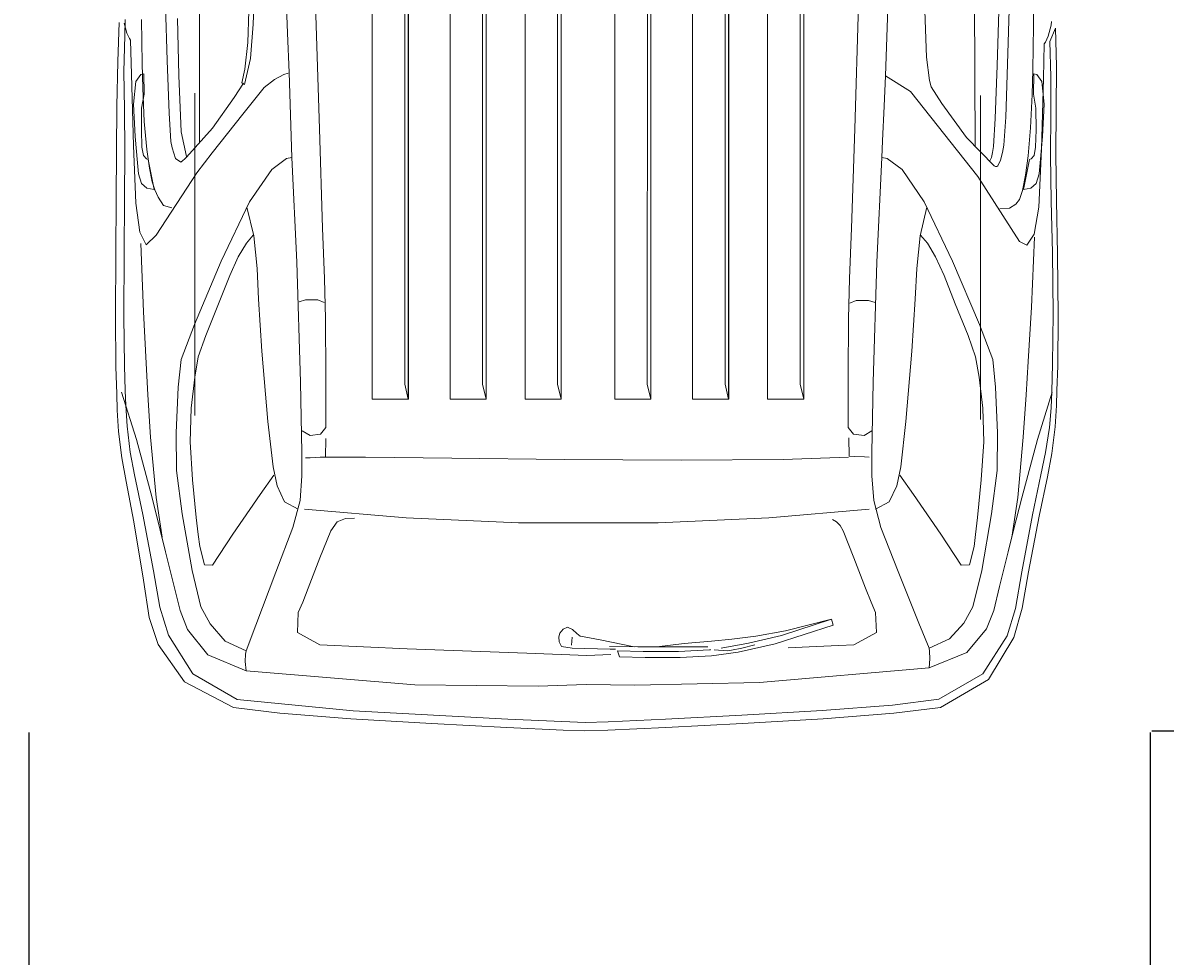
# Model space of a CAD drawing. Units: inches. Extents: x 37 to 706, y -568 to 110.
# Tile 3 of 24: x 126 to 171, y -450 to -413. Entities that reach past the tile are written whole.
import ezdxf

# ---------------------------------------------------------------- set-up
doc = ezdxf.new("R2010")
doc.units = ezdxf.units.IN
doc.header["$MEASUREMENT"] = 0
for name, color, linetype, lineweight in [('A-ANNO-DIMS', 2, 'Continuous', 18), ('A-SITE-VEHI', 8, 'Continuous', 13), ('A-WALL-PATT', 252, 'Continuous', 13)]:
    doc.layers.add(name, color=color, linetype=linetype, lineweight=lineweight)
doc.styles.get("Standard").update_dxf_attribs({"font": 'arial.ttf'})
doc.dimstyles.get("Standard").update_dxf_attribs({"dimtxt": 0.18, "dimasz": 0.18, "dimexe": 0.18, "dimexo": 0.0625, "dimgap": 0.09, "dimtad": 0, "dimtih": 1, "dimtoh": 1, "dimdec": 0, "dimzin": 0, "dimdsep": 46, "dimlunit": 3, "dimtxsty": 'Standard', "dimcen": 0.09, "dimadec": 0, "dimazin": 0, "dimtfac": 1, "dimtdec": 0, "dimtofl": 0, "dimtmove": 0, "dimatfit": 3, "dimfxl": 1, "dimtolj": 1, "dimtzin": 0, "dimarcsym": 0})

# ---------------------------------------------------------------- blocks, each defined once
blk = doc.blocks.new('CAR-SEDAN-PLAN')
for p, q in [((13.604, 13.133), (13.604, 50.661)), ((14.891, 13.73), (14.905, 50.543)), ((15.034, 50.661), (15.034, 13.133)), ((15.035, 50.661), (15.035, 13.133)), ((16.686, 13.133), (16.686, 50.661)), ((17.973, 13.73), (17.987, 50.543)), ((18.115, 50.661), (18.115, 13.133)), ((18.117, 50.661), (18.117, 13.133)), ((19.657, 13.133), (19.657, 50.661)), ((20.944, 13.73), (20.958, 50.543)), ((21.087, 50.661), (21.087, 13.133)), ((21.088, 50.661), (21.088, 13.133)), ((23.212, 13.133), (23.212, 50.661)), ((24.499, 13.73), (24.513, 50.543)), ((24.642, 50.661), (24.642, 13.133)), ((24.643, 50.661), (24.643, 13.133)), ((26.294, 13.133), (26.294, 50.661)), ((27.581, 13.73), (27.595, 50.543)), ((27.723, 50.661), (27.723, 13.133)), ((27.725, 50.661), (27.725, 13.133)), ((29.265, 13.133), (29.265, 50.661)), ((30.553, 13.73), (30.567, 50.543)), ((30.696, 50.661), (30.696, 13.133)), ((34.17, 32.694), (34.002, 27.855)), ((10.065, 32.102), (10.25, 27.635)), ((6.755, 31.469), (6.762, 26.153)), ((39.857, 31.627), (39.796, 27.924)), ((37.457, 31.221), (37.48, 25.971)), ((5.415, 28.71), (5.486, 26.554)), ((8.919, 28.667), (8.894, 27.992)), ((11.511, 23.847), (11.355, 28.753)), ((32.718, 23.847), (32.874, 28.753)), ((35.501, 28.522), (35.566, 26.682)), ((38.84, 28.558), (38.769, 26.402)), ((3.52, 26.505), (3.579, 28.059)), ((3.815, 28.178), (3.801, 27.531)), ((4.464, 28.172), (4.492, 26.437)), ((5.892, 28.219), (5.946, 25.954)), ((8.671, 27.267), (8.713, 28.508)), ((38.427, 28.503), (38.356, 26.347)), ((40.498, 27.951), (40.519, 28.091)), ((3.88, 27.64), (3.771, 28.026)), ((3.984, 27.426), (3.88, 27.64)), ((8.894, 27.992), (8.788, 26.636)), ((10.25, 27.635), (10.317, 26.081)), ((34.002, 27.855), (33.939, 25.939)), ((39.796, 27.924), (39.768, 26.188)), ((40.387, 27.519), (40.498, 27.951)), ((40.449, 27.298), (40.675, 27.828)), ((40.675, 27.828), (40.709, 26.308)), ((3.801, 27.531), (3.77, 26.116)), ((4.03, 27.36), (3.984, 27.426)), ((4.062, 25.992), (4.03, 27.36)), ((8.558, 26.208), (8.671, 27.267)), ((40.194, 25.84), (40.225, 27.208)), ((40.225, 27.208), (40.276, 27.281)), ((40.276, 27.281), (40.387, 27.519)), ((40.488, 25.901), (40.449, 27.298)), ((3.484, 24.748), (3.52, 26.505)), ((4.492, 26.437), (4.514, 25.45)), ((5.486, 26.554), (5.557, 24.461)), ((8.788, 26.636), (8.548, 25.606)), ((35.566, 26.682), (35.686, 25.757)), ((38.356, 26.347), (38.285, 24.254)), ((38.769, 26.402), (38.698, 24.309)), ((40.709, 26.308), (40.697, 24.613)), ((3.77, 26.116), (3.787, 24.613)), ((4.141, 23.187), (4.062, 25.992)), ((4.44, 26.001), (4.24, 25.718)), ((4.551, 26.018), (4.44, 26.001)), ((4.571, 25.221), (4.551, 26.018)), ((5.946, 25.954), (6.033, 23.727)), ((6.762, 26.153), (6.765, 23.311)), ((8.437, 25.661), (8.558, 26.208)), ((9.729, 25.804), (9.322, 25.478)), ((10.107, 25.994), (9.729, 25.804)), ((10.273, 26.055), (10.107, 25.994)), ((10.317, 26.081), (10.426, 22.71)), ((33.939, 25.939), (33.885, 24.736)), ((33.939, 25.939), (34.933, 25.326)), ((37.48, 25.971), (37.49, 23.159)), ((39.768, 26.188), (39.746, 25.202)), ((39.796, 25.221), (39.816, 26.018)), ((39.816, 26.018), (39.928, 26.001)), ((39.928, 26.001), (40.128, 25.718)), ((40.115, 23.036), (40.194, 25.84)), ((40.485, 24.433), (40.488, 25.901)), ((4.24, 25.718), (4.151, 24.827)), ((4.514, 25.45), (4.576, 24.132)), ((8.505, 25.655), (8.139, 25.088)), ((8.548, 25.606), (8.437, 25.661)), ((9.322, 25.478), (8.474, 24.429)), ((35.686, 25.757), (35.75, 25.503)), ((35.75, 25.503), (36.174, 24.851)), ((40.128, 25.718), (40.217, 24.827)), ((4.47, 24.664), (4.571, 25.221)), ((6.579, 25.262), (6.579, 12.495)), ((8.139, 25.088), (7.271, 23.868)), ((34.933, 25.326), (37.597, 21.952)), ((37.699, 25.17), (37.699, 12.334)), ((39.746, 25.202), (39.684, 23.884)), ((39.897, 24.664), (39.796, 25.221)), ((3.472, 22.96), (3.484, 24.748)), ((3.787, 24.613), (3.803, 22.96)), ((4.151, 24.827), (4.216, 23.545)), ((4.466, 23.8), (4.47, 24.664)), ((5.557, 24.461), (5.628, 23.347)), ((33.885, 24.736), (33.823, 23.365)), ((36.174, 24.851), (37.15, 23.504)), ((39.901, 23.8), (39.897, 24.664)), ((40.217, 24.827), (40.151, 23.545)), ((40.697, 24.613), (40.683, 22.854)), ((4.576, 24.132), (4.669, 23.027)), ((8.474, 24.429), (7.27, 22.892)), ((38.285, 24.254), (38.214, 23.14)), ((38.698, 24.309), (38.627, 23.195)), ((40.477, 22.799), (40.485, 24.433)), ((4.216, 23.545), (4.303, 22.495)), ((4.482, 23.116), (4.466, 23.8)), ((6.033, 23.727), (6.25, 22.744)), ((7.271, 23.868), (6.252, 22.718)), ((11.64, 19.914), (11.511, 23.847)), ((32.59, 19.914), (32.718, 23.847)), ((39.684, 23.884), (39.591, 22.779)), ((39.885, 23.116), (39.901, 23.8)), ((40.151, 23.545), (40.064, 22.495)), ((4.243, 20.896), (4.141, 23.187)), ((4.546, 22.789), (4.482, 23.116)), ((5.628, 23.347), (5.675, 23.096)), ((5.675, 23.096), (5.809, 22.664)), ((33.823, 23.365), (33.793, 22.71)), ((37.15, 23.504), (38.236, 22.378)), ((38.214, 23.14), (38.178, 22.908)), ((38.627, 23.195), (38.57, 22.906)), ((39.821, 22.789), (39.885, 23.116)), ((3.463, 21.075), (3.472, 22.96)), ((3.803, 22.96), (3.793, 21.075)), ((4.666, 22.658), (4.546, 22.789)), ((4.73, 22.634), (4.666, 22.658)), ((4.669, 23.027), (4.776, 22.289)), ((4.964, 21.437), (4.73, 22.634)), ((5.809, 22.664), (6.019, 22.53)), ((6.095, 22.587), (6.173, 22.65)), ((6.173, 22.65), (6.252, 22.718)), ((7.27, 22.892), (6.658, 22.104)), ((10.213, 22.669), (9.627, 22.239)), ((10.426, 22.71), (10.213, 22.669)), ((10.426, 22.71), (10.623, 18.569)), ((33.793, 22.71), (33.596, 18.569)), ((33.793, 22.71), (34.007, 22.669)), ((34.007, 22.669), (34.593, 22.239)), ((38.142, 22.707), (38.056, 22.552)), ((38.178, 22.908), (38.142, 22.707)), ((38.57, 22.906), (38.496, 22.598)), ((39.404, 21.437), (39.637, 22.634)), ((39.591, 22.779), (39.479, 22.007)), ((39.637, 22.634), (39.702, 22.658)), ((39.702, 22.658), (39.821, 22.789)), ((40.012, 20.744), (40.115, 23.036)), ((40.502, 20.982), (40.477, 22.799)), ((40.683, 22.854), (40.709, 20.996)), ((4.303, 22.495), (4.347, 22.059)), ((4.776, 22.289), (4.883, 21.74)), ((6.019, 22.53), (6.095, 22.587)), ((9.627, 22.239), (8.747, 20.959)), ((34.593, 22.239), (35.473, 20.959)), ((38.236, 22.378), (38.293, 22.351)), ((38.293, 22.351), (38.344, 22.355)), ((38.344, 22.355), (38.389, 22.385)), ((38.496, 22.598), (38.389, 22.385)), ((40.064, 22.495), (40.02, 22.059)), ((4.347, 22.059), (4.458, 21.676)), ((4.883, 21.74), (4.989, 21.429)), ((6.658, 22.104), (5.04, 19.635)), ((37.597, 21.952), (39.239, 19.387)), ((39.479, 22.007), (39.364, 21.397)), ((40.02, 22.059), (39.909, 21.676)), ((4.458, 21.676), (4.673, 21.491)), ((4.673, 21.491), (4.964, 21.437)), ((4.989, 21.429), (5.122, 21.136)), ((39.364, 21.397), (39.252, 21.052)), ((39.695, 21.491), (39.404, 21.437)), ((39.909, 21.676), (39.695, 21.491)), ((3.446, 18.903), (3.463, 21.075)), ((3.793, 21.075), (3.776, 18.903)), ((4.396, 19.749), (4.243, 20.896)), ((5.122, 21.136), (5.335, 20.805)), ((8.747, 20.959), (7.622, 18.6)), ((35.473, 20.959), (36.598, 18.6)), ((39.099, 20.862), (38.843, 20.707)), ((39.252, 21.052), (39.099, 20.862)), ((40.548, 18.939), (40.502, 20.982)), ((40.709, 20.996), (40.757, 18.876)), ((5.335, 20.805), (5.672, 20.722)), ((8.64, 20.745), (8.911, 19.602)), ((35.58, 20.745), (35.309, 19.602)), ((38.843, 20.707), (38.468, 20.681)), ((39.822, 19.677), (40.012, 20.744)), ((11.712, 17.922), (11.64, 19.914)), ((32.517, 17.922), (32.59, 19.914)), ((4.655, 19.245), (4.396, 19.749)), ((5.04, 19.635), (4.655, 19.245)), ((8.89, 19.637), (8.625, 19.316)), ((8.911, 19.602), (9.047, 18.315)), ((35.309, 19.602), (35.172, 18.315)), ((35.33, 19.637), (35.595, 19.316)), ((39.532, 19.233), (39.822, 19.677)), ((39.844, 19.553), (39.718, 16.784)), ((4.434, 19.305), (4.545, 16.6)), ((8.625, 19.316), (8.297, 18.78)), ((35.595, 19.316), (35.923, 18.78)), ((39.239, 19.387), (39.532, 19.233)), ((3.437, 16.422), (3.446, 18.903)), ((3.776, 18.903), (3.767, 16.422)), ((7.622, 18.6), (6.561, 16.09)), ((8.297, 18.78), (7.961, 18.03)), ((10.623, 18.569), (10.765, 13.809)), ((33.596, 18.569), (33.455, 13.809)), ((35.923, 18.78), (36.259, 18.03)), ((36.598, 18.6), (37.659, 16.09)), ((40.573, 16.526), (40.548, 18.939)), ((40.757, 18.876), (40.783, 16.422)), ((9.047, 18.315), (9.104, 17.101)), ((35.172, 18.315), (35.115, 17.101)), ((7.961, 18.03), (7.517, 16.918)), ((11.752, 16.319), (11.712, 17.922)), ((32.477, 16.319), (32.517, 17.922)), ((36.259, 18.03), (36.702, 16.918)), ((7.517, 16.918), (7.011, 15.663)), ((9.104, 17.101), (9.236, 15.044)), ((10.707, 16.994), (10.967, 17.077)), ((10.967, 17.077), (11.449, 17.073)), ((11.449, 17.073), (11.705, 16.973)), ((32.78, 17.046), (32.525, 16.946)), ((33.262, 17.05), (32.78, 17.046)), ((33.522, 16.966), (33.262, 17.05)), ((35.115, 17.101), (34.983, 15.044)), ((36.702, 16.918), (37.209, 15.663)), ((39.718, 16.784), (39.589, 14.629)), ((3.453, 14.417), (3.437, 16.422)), ((3.767, 16.422), (3.785, 14.465)), ((4.545, 16.6), (4.646, 14.565)), ((11.771, 14.081), (11.752, 16.319)), ((32.458, 14.081), (32.477, 16.319)), ((40.555, 14.519), (40.573, 16.526)), ((40.783, 16.422), (40.764, 14.465)), ((6.561, 16.09), (6.031, 14.707)), ((37.659, 16.09), (38.188, 14.707)), ((7.011, 15.663), (6.71, 14.814)), ((37.209, 15.663), (37.509, 14.814)), ((9.236, 15.044), (9.472, 12.249)), ((34.983, 15.044), (34.748, 12.249)), ((4.646, 14.565), (4.709, 13.313)), ((6.031, 14.707), (5.922, 13.615)), ((6.71, 14.814), (6.571, 14.015)), ((37.509, 14.814), (37.648, 14.015)), ((38.188, 14.707), (38.298, 13.615)), ((39.589, 14.629), (39.51, 13.313)), ((40.522, 13.447), (40.555, 14.519)), ((3.483, 13.349), (3.453, 14.417)), ((3.785, 14.465), (3.82, 13.484)), ((11.772, 12.018), (11.771, 14.081)), ((32.458, 12.018), (32.458, 14.081)), ((40.764, 14.465), (40.73, 13.484)), ((5.922, 13.615), (5.844, 11.809)), ((6.571, 14.015), (6.432, 12.779)), ((10.765, 13.809), (10.819, 11.026)), ((15.034, 13.133), (14.891, 13.73)), ((18.115, 13.133), (17.973, 13.73)), ((21.087, 13.133), (20.944, 13.73)), ((24.642, 13.133), (24.499, 13.73)), ((27.723, 13.133), (27.581, 13.73)), ((30.696, 13.133), (30.553, 13.73)), ((33.455, 13.809), (33.4, 11.026)), ((37.648, 14.015), (37.787, 12.779)), ((38.298, 13.615), (38.376, 11.809)), ((3.499, 12.702), (3.483, 13.349)), ((3.673, 13.421), (4.262, 11.543)), ((3.82, 13.484), (3.838, 12.885)), ((4.709, 13.313), (4.826, 11.635)), ((15.035, 13.133), (13.604, 13.133)), ((18.117, 13.133), (16.686, 13.133)), ((21.088, 13.133), (19.657, 13.133)), ((24.643, 13.133), (23.212, 13.133)), ((27.725, 13.133), (26.294, 13.133)), ((30.696, 13.133), (29.265, 13.133)), ((39.51, 13.313), (39.394, 11.635)), ((40.546, 13.421), (39.958, 11.543)), ((40.504, 12.798), (40.522, 13.447)), ((40.73, 13.484), (40.711, 12.885)), ((3.552, 11.862), (3.499, 12.702)), ((3.838, 12.885), (3.891, 12.073)), ((6.432, 12.779), (6.389, 11.455)), ((37.787, 12.779), (37.831, 11.455)), ((40.436, 12.011), (40.504, 12.798)), ((40.711, 12.885), (40.658, 12.044)), ((9.472, 12.249), (9.676, 10.455)), ((34.748, 12.249), (34.544, 10.455)), ((3.686, 10.809), (3.552, 11.862)), ((3.891, 12.073), (4.021, 11.046)), ((5.844, 11.809), (5.853, 10.312)), ((10.833, 11.88), (11.14, 11.695)), ((11.56, 11.754), (11.772, 12.018)), ((32.669, 11.754), (32.458, 12.018)), ((33.396, 11.88), (33.089, 11.695)), ((38.376, 11.809), (38.367, 10.312)), ((40.277, 11.029), (40.436, 12.011)), ((40.658, 12.044), (40.524, 10.992)), ((4.262, 11.543), (4.883, 9.236)), ((4.826, 11.635), (5.045, 9.251)), ((6.389, 11.455), (6.488, 9.945)), ((11.14, 11.695), (11.56, 11.754)), ((11.772, 11.581), (11.748, 10.848)), ((32.479, 11.611), (32.503, 10.878)), ((33.089, 11.695), (32.669, 11.754)), ((37.831, 11.455), (37.732, 9.945)), ((39.394, 11.635), (39.174, 9.251)), ((39.958, 11.543), (39.337, 9.236)), ((4.021, 11.046), (4.191, 10.136)), ((10.819, 11.026), (10.822, 10.099)), ((32.503, 10.878), (32.714, 10.869)), ((32.714, 10.869), (33.101, 10.852)), ((33.4, 11.026), (33.398, 10.099)), ((40.092, 10.143), (40.277, 11.029)), ((40.524, 10.992), (40.35, 10.059)), ((3.861, 9.877), (3.686, 10.809)), ((9.676, 10.455), (9.84, 9.71)), ((11.15, 10.821), (10.962, 10.812)), ((11.536, 10.839), (11.15, 10.821)), ((11.748, 10.848), (11.536, 10.839)), ((13.334, 10.84), (11.748, 10.848)), ((16.76, 10.8), (13.334, 10.84)), ((21.205, 10.754), (16.76, 10.8)), ((25.852, 10.729), (21.205, 10.754)), ((29.881, 10.751), (25.852, 10.729)), ((32.471, 10.848), (29.881, 10.751)), ((33.101, 10.852), (33.289, 10.843)), ((34.544, 10.455), (34.38, 9.71)), ((4.191, 10.136), (4.515, 8.572)), ((5.853, 10.312), (6.079, 8.596)), ((9.169, 9.358), (9.711, 10.133)), ((10.822, 10.099), (10.745, 9.132)), ((33.398, 10.099), (33.475, 9.132)), ((35.051, 9.358), (34.508, 10.133)), ((38.367, 10.312), (38.141, 8.596)), ((39.767, 8.563), (40.092, 10.143)), ((40.35, 10.059), (40.028, 8.506)), ((4.16, 8.275), (3.861, 9.877)), ((6.488, 9.945), (6.635, 8.451)), ((9.84, 9.71), (10.131, 9.068)), ((34.38, 9.71), (34.089, 9.068)), ((37.732, 9.945), (37.585, 8.451)), ((4.883, 9.236), (5.21, 7.954)), ((5.045, 9.251), (5.281, 7.668)), ((8.087, 7.788), (9.169, 9.358)), ((10.131, 9.068), (10.676, 8.776)), ((10.745, 9.132), (10.462, 8.061)), ((33.475, 9.132), (33.758, 8.061)), ((34.089, 9.068), (33.543, 8.776)), ((36.133, 7.788), (35.051, 9.358)), ((39.174, 9.251), (38.939, 7.668)), ((39.337, 9.236), (39.01, 7.954)), ((14.948, 8.438), (10.926, 8.776)), ((33.293, 8.776), (29.309, 8.438)), ((4.542, 5.974), (4.16, 8.275)), ((4.515, 8.572), (4.943, 6.346)), ((6.079, 8.596), (6.472, 6.347)), ((6.635, 8.451), (6.71, 7.775)), ((11.963, 7.918), (12.22, 8.276)), ((12.22, 8.276), (12.546, 8.416)), ((12.546, 8.416), (12.908, 8.42)), ((19.398, 8.244), (14.948, 8.438)), ((22.181, 8.24), (19.398, 8.244)), ((24.927, 8.244), (22.181, 8.24)), ((29.309, 8.438), (24.927, 8.244)), ((31.842, 8.368), (31.999, 8.276)), ((31.999, 8.276), (32.139, 8.129)), ((37.585, 8.451), (37.509, 7.775)), ((38.141, 8.596), (37.748, 6.347)), ((39.34, 6.307), (39.767, 8.563)), ((40.028, 8.506), (39.603, 6.295)), ((5.21, 7.954), (5.421, 7.098)), ((6.71, 7.775), (6.771, 7.309)), ((7.282, 6.56), (8.087, 7.788)), ((10.462, 8.061), (9.79, 6.285)), ((11.533, 6.853), (11.963, 7.918)), ((32.139, 8.129), (32.257, 7.918)), ((32.257, 7.918), (32.687, 6.853)), ((33.758, 8.061), (34.442, 6.313)), ((36.938, 6.56), (36.133, 7.788)), ((37.509, 7.775), (37.448, 7.309)), ((39.01, 7.954), (38.798, 7.098)), ((6.771, 7.309), (6.959, 6.574)), ((37.448, 7.309), (37.261, 6.574)), ((5.421, 7.098), (5.76, 5.725)), ((11.071, 5.66), (11.533, 6.853)), ((32.687, 6.853), (33.149, 5.66)), ((38.798, 7.098), (38.459, 5.725)), ((4.943, 6.346), (5.195, 4.901)), ((6.472, 6.347), (6.817, 4.917)), ((6.959, 6.574), (7.282, 6.56)), ((37.261, 6.574), (36.938, 6.56)), ((37.748, 6.347), (37.402, 4.917)), ((4.77, 4.491), (4.542, 5.974)), ((9.79, 6.285), (8.99, 4.184)), ((34.442, 6.313), (35.263, 4.266)), ((39.087, 4.847), (39.34, 6.307)), ((39.603, 6.295), (39.352, 4.86)), ((5.76, 5.725), (5.996, 4.774)), ((10.855, 5.095), (11.071, 5.66)), ((33.149, 5.66), (33.365, 5.095)), ((38.459, 5.725), (38.224, 4.774)), ((10.674, 4.684), (10.855, 5.095)), ((33.365, 5.095), (33.546, 4.684)), ((5.195, 4.901), (5.531, 3.798)), ((5.996, 4.774), (6.288, 4.02)), ((6.817, 4.917), (7.185, 4.242)), ((10.643, 3.899), (10.674, 4.684)), ((33.546, 4.684), (33.576, 3.899)), ((37.402, 4.917), (37.046, 4.27)), ((38.224, 4.774), (37.943, 4.048)), ((38.757, 3.761), (39.087, 4.847)), ((39.352, 4.86), (39.023, 3.695)), ((5.125, 3.422), (4.77, 4.491)), ((7.185, 4.242), (7.784, 3.56)), ((8.99, 4.184), (8.604, 3.17)), ((21.162, 4.032), (21.341, 4.104)), ((21.341, 4.104), (21.538, 4.014)), ((29.573, 3.454), (31.866, 4.183)), ((31.793, 4.421), (29.822, 3.785)), ((31.793, 4.421), (29.98, 3.966)), ((31.866, 4.183), (31.793, 4.421)), ((35.263, 4.266), (35.662, 3.281)), ((37.046, 4.27), (36.47, 3.641)), ((5.531, 3.798), (6.501, 2.261)), ((6.288, 4.02), (7.089, 3.02)), ((11.534, 3.416), (10.643, 3.899)), ((20.997, 3.733), (21.034, 3.871)), ((21.004, 3.524), (20.997, 3.733)), ((21.034, 3.871), (21.162, 4.032)), ((21.499, 3.391), (21.521, 3.714)), ((21.538, 4.014), (21.716, 3.853)), ((21.716, 3.853), (21.845, 3.754)), ((22.004, 3.727), (21.845, 3.754)), ((22.637, 3.606), (22.004, 3.727)), ((27.853, 3.637), (27.049, 3.559)), ((28.803, 3.753), (27.853, 3.637)), ((29.822, 3.785), (28.511, 3.471)), ((29.98, 3.966), (28.803, 3.753)), ((33.576, 3.899), (32.686, 3.416)), ((36.47, 3.641), (35.662, 3.281)), ((37.943, 4.048), (37.164, 3.102)), ((37.799, 2.256), (38.757, 3.761)), ((39.023, 3.695), (38.022, 2.04)), ((6.173, 1.944), (5.125, 3.422)), ((7.784, 3.56), (8.604, 3.17)), ((8.604, 3.17), (8.588, 3.046)), ((14.99, 3.257), (11.534, 3.416)), ((19.725, 3.075), (14.99, 3.257)), ((21.096, 3.341), (21.004, 3.524)), ((21.524, 3.276), (21.096, 3.341)), ((23.024, 3.239), (21.524, 3.276)), ((23.982, 3.332), (22.637, 3.606)), ((24.129, 3.334), (23.01, 3.34)), ((23.236, 3.237), (23.024, 3.239)), ((24.339, 3.147), (23.324, 3.177)), ((23.324, 3.177), (23.396, 2.94)), ((25.943, 3.33), (24.129, 3.334)), ((25.968, 3.461), (24.882, 3.334)), ((26.968, 3.215), (25.734, 3.146)), ((26.893, 3.328), (25.943, 3.33)), ((27.049, 3.559), (25.968, 3.461)), ((26.981, 3.216), (26.968, 3.215)), ((26.995, 3.218), (26.981, 3.216)), ((27.01, 3.22), (26.995, 3.218)), ((27.673, 3.169), (27.15, 3.209)), ((28.511, 3.471), (27.428, 3.283)), ((27.835, 3.2), (27.673, 3.169)), ((28.24, 3.283), (27.835, 3.2)), ((28.095, 3.12), (29.573, 3.454)), ((28.765, 3.406), (28.24, 3.283)), ((31.193, 3.34), (30.088, 3.293)), ((32.083, 3.382), (31.193, 3.34)), ((32.686, 3.416), (32.083, 3.382)), ((35.662, 3.281), (35.678, 3.156)), ((7.089, 3.02), (8.604, 2.384)), ((8.588, 3.046), (8.572, 2.747)), ((8.572, 2.747), (8.604, 2.384)), ((22.11, 2.987), (19.725, 3.075)), ((23.061, 3.022), (22.11, 2.987)), ((23.396, 2.94), (24.411, 2.909)), ((25.734, 3.146), (24.339, 3.147)), ((24.411, 2.909), (25.806, 2.909)), ((25.806, 2.909), (27.04, 2.977)), ((27.04, 2.977), (28.095, 3.12)), ((37.164, 3.102), (35.662, 2.494)), ((35.694, 2.857), (35.662, 2.494)), ((35.678, 3.156), (35.694, 2.857)), ((15.288, 1.831), (8.604, 2.384)), ((35.662, 2.494), (28.947, 1.913)), ((8.107, 0.932), (6.173, 1.944)), ((6.501, 2.261), (8.259, 1.242)), ((20.178, 1.778), (15.288, 1.831)), ((22.074, 1.844), (20.178, 1.778)), ((24.001, 1.806), (22.074, 1.844)), ((28.947, 1.913), (24.001, 1.806)), ((36.048, 1.256), (37.799, 2.256)), ((38.022, 2.04), (36.112, 0.932)), ((9.948, 0.701), (8.107, 0.932)), ((8.259, 1.242), (12.855, 0.801)), ((31.426, 0.81), (34.217, 1.026)), ((34.217, 1.026), (36.048, 1.256)), ((36.112, 0.932), (34.271, 0.701)), ((12.757, 0.482), (9.948, 0.701)), ((15.951, 0.29), (12.757, 0.482)), ((12.855, 0.801), (18.978, 0.464)), ((18.978, 0.464), (22.045, 0.33)), ((22.946, 0.366), (25.227, 0.467)), ((25.227, 0.467), (28.251, 0.62)), ((28.251, 0.62), (31.426, 0.81)), ((31.463, 0.482), (28.269, 0.29)), ((34.271, 0.701), (31.463, 0.482)), ((18.943, 0.137), (15.951, 0.29)), ((21.163, 0.036), (18.943, 0.137)), ((22.032, 0), (21.163, 0.036)), ((22.941, 0.036), (22.032, 0)), ((22.045, 0.33), (22.946, 0.366)), ((25.236, 0.137), (22.941, 0.036)), ((28.269, 0.29), (25.236, 0.137))]:
    blk.add_line(p, q)
blk = doc.blocks.new('*D29')
at = {"layer": 'A-ANNO-DIMS', "color": 0, "lineweight": -2, "transparency": 16777216}
for p, q in [((170.913, -348.62), (184.856, -348.62)), ((184.676, -348.8), (184.676, -394.522)), ((184.676, -440.609), (184.676, -394.888)), ((170.913, -440.789), (184.856, -440.789))]:
    blk.add_line(p, q, dxfattribs=at)
at = {"layer": 'A-ANNO-DIMS', "color": 0, "transparency": 16777216}
for points in [[(184.646, -348.8), (184.706, -348.8), (184.676, -348.62)], [(184.646, -440.609), (184.706, -440.609), (184.676, -440.789)]]:
    blk.add_solid(points, dxfattribs=at)
at = {"layer": 'Defpoints', "color": 0, "transparency": 16777216}
for p in [(170.851, -348.62), (184.676, -348.62), (170.851, -440.789)]:
    blk.add_point(p, dxfattribs=at)
at = {"layer": 'A-ANNO-DIMS', "color": 0, "transparency": 16777216, "insert": (184.676, -394.705), "char_height": 0.18, "attachment_point": 5}
blk.add_mtext('\\A1;CAR 7\'-8" TYP.', dxfattribs=at)
blk = doc.blocks.new('*D30')
at = {"layer": 'A-ANNO-DIMS', "color": 0, "lineweight": -2, "transparency": 16777216}
for p, q in [((126.431, -440.852), (126.431, -454.795)), ((170.851, -440.852), (170.851, -454.795)), ((126.611, -454.615), (147.793, -454.615)), ((170.671, -454.615), (149.489, -454.615))]:
    blk.add_line(p, q, dxfattribs=at)
at = {"layer": 'A-ANNO-DIMS', "color": 0, "transparency": 16777216}
for points in [[(126.611, -454.585), (126.611, -454.645), (126.431, -454.615)], [(170.671, -454.585), (170.671, -454.645), (170.851, -454.615)]]:
    blk.add_solid(points, dxfattribs=at)
at = {"layer": 'Defpoints', "color": 0, "transparency": 16777216}
for p in [(126.431, -440.789), (170.851, -440.789), (170.851, -454.615)]:
    blk.add_point(p, dxfattribs=at)
at = {"layer": 'A-ANNO-DIMS', "color": 0, "transparency": 16777216, "insert": (148.641, -454.615), "char_height": 0.18, "attachment_point": 5}
blk.add_mtext('\\A1;3\'-8 1/2" TYP.', dxfattribs=at)

msp = doc.modelspace()

# ---------------------------------------------------------------- hatches: boundary and pattern name
at = {"layer": 'A-WALL-PATT'}
h = msp.add_hatch(color=256, dxfattribs=at)
h.dxf.hatch_style = 1
h.paths.add_polyline_path([(220.958, -351.708), (211.958, -351.708), (211.958, -513.708), (254.958, -513.708), (254.958, -504.708), (220.958, -504.708)], flags=17)
h.paths.add_polyline_path([(220.958, -294.708), (211.958, -294.708), (211.958, -303.708), (220.958, -303.708)], flags=17)
h.paths.add_polyline_path([(175.958, -294.708), (155.871, -294.708), (155.871, -303.708), (155.958, -303.708), (175.958, -303.708)], flags=17)
h.paths.add_polyline_path([(220.958, -16.708), (211.958, -16.708), (211.958, -142.708), (220.958, -142.708)], flags=17)
h.paths.add_polyline_path([(357.958, 51.292), (78.958, 51.292), (78.958, -513.708), (87.958, -513.708), (87.958, -303.708), (95.871, -303.708), (95.871, -294.708), (87.958, -294.708), (87.958, -142.708), (187.958, -142.708), (187.958, -133.708), (87.958, -133.708), (87.958, -25.708), (106.958, -25.708), (106.958, -16.708), (87.958, -16.708), (87.958, 42.292), (348.958, 42.292), (348.958, 17.129), (348.958, -133.708), (246.958, -133.708), (246.958, -142.708), (348.958, -142.708), (348.958, -294.708), (251.958, -294.708), (251.958, -303.708), (348.958, -303.708), (348.958, -351.708), (260.958, -351.708), (260.958, -329.708), (251.958, -329.708), (251.958, -360.708), (327.446, -360.708), (348.958, -360.708), (348.958, -504.708), (314.958, -504.708), (314.958, -513.708), (357.958, -513.708)])
h.paths.add_polyline_path([(416.958, -303.708), (402.958, -303.708), (402.958, -151.708), (478.958, -151.708), (478.958, -142.708), (402.958, -142.708), (402.958, -22.708), (409.958, -22.708), (409.958, -13.708), (402.958, -13.708), (402.958, 42.292), (663.958, 42.292), (663.958, -303.708), (566.958, -303.708), (566.958, -312.708), (663.958, -312.708), (663.958, -360.708), (575.958, -360.708), (575.958, -338.708), (566.958, -338.708), (566.958, -360.708), (566.958, -369.708), (642.446, -369.708), (663.958, -369.708), (663.958, -513.708), (629.958, -513.708), (629.958, -522.708), (672.958, -522.708), (672.958, 51.292), (393.958, 51.292), (393.958, -522.708), (402.958, -522.708), (402.958, -312.708), (416.958, -312.708)])
h.paths.add_polyline_path([(490.958, -303.708), (476.958, -303.708), (476.958, -312.708), (490.958, -312.708)], flags=17)
h.paths.add_polyline_path([(535.958, -303.708), (526.958, -303.708), (526.958, -312.708), (535.958, -312.708)], flags=17)
h.paths.add_polyline_path([(535.958, -369.708), (526.958, -369.708), (526.958, -522.708), (569.958, -522.708), (569.958, -513.708), (535.958, -513.708)], flags=17)
h.paths.add_polyline_path([(511.958, -13.708), (502.958, -13.708), (502.958, -151.708), (511.958, -151.708)], flags=17)
h.paths.add_polyline_path([(651.539, -142.708), (651.539, -120.181), (642.539, -120.181), (642.539, -142.708), (550.539, -142.708), (550.539, -120.708), (541.539, -120.708), (541.539, -142.708), (537.958, -142.708), (537.958, -151.708), (651.539, -151.708)], flags=17)
h.paths.add_polyline_path([(651.539, -85.708), (541.539, -85.708), (541.539, -94.708), (651.539, -94.708)], flags=17)
h.paths.add_polyline_path([(476.958, -13.708), (469.958, -13.708), (469.958, -22.708), (476.958, -22.708)], flags=17)
h.paths.add_polyline_path([(185.958, -16.708), (166.958, -16.708), (166.958, -25.708), (185.958, -25.708)], flags=17)
h.paths.add_polyline_path([(168.909, -414.719), (214.621, -414.719), (214.621, -392.33), (168.909, -392.33)], flags=25)

# ---------------------------------------------------------------- block references
at = {"layer": 'A-SITE-VEHI'}
msp.add_blockref('CAR-SEDAN-PLAN', (126.431, -440.789), dxfattribs=at)

# ---------------------------------------------------------------- dimensions: what is measured, and where the dimension line sits
at = {"layer": 'A-ANNO-DIMS'}
dim = msp.add_linear_dim(base=(184.676, -348.62), p1=(170.851, -440.789), p2=(170.851, -348.62), angle=90, text='CAR <> TYP.', dimstyle='Standard', override={"dimdec": 1, "dimlfac": 1, "dimrnd": 0, "dimzin": 1, "dimdsep": 46, "dimlunit": 4, "dimfrac": 2}, dxfattribs=at)
dim.commit()
dim.dimension.update_dxf_attribs({"geometry": '*D29', "text_midpoint": (184.676, -394.705)})
dim = msp.add_linear_dim(base=(170.851, -454.615), p1=(126.431, -440.789), p2=(170.851, -440.789), text='<> TYP.', dimstyle='Standard', override={"dimdec": 1, "dimlfac": 1, "dimrnd": 0, "dimzin": 1, "dimdsep": 46, "dimlunit": 4, "dimfrac": 2}, dxfattribs=at)
dim.commit()
dim.dimension.update_dxf_attribs({"geometry": '*D30', "text_midpoint": (148.641, -454.615)})

doc.saveas('drawing.dxf')
